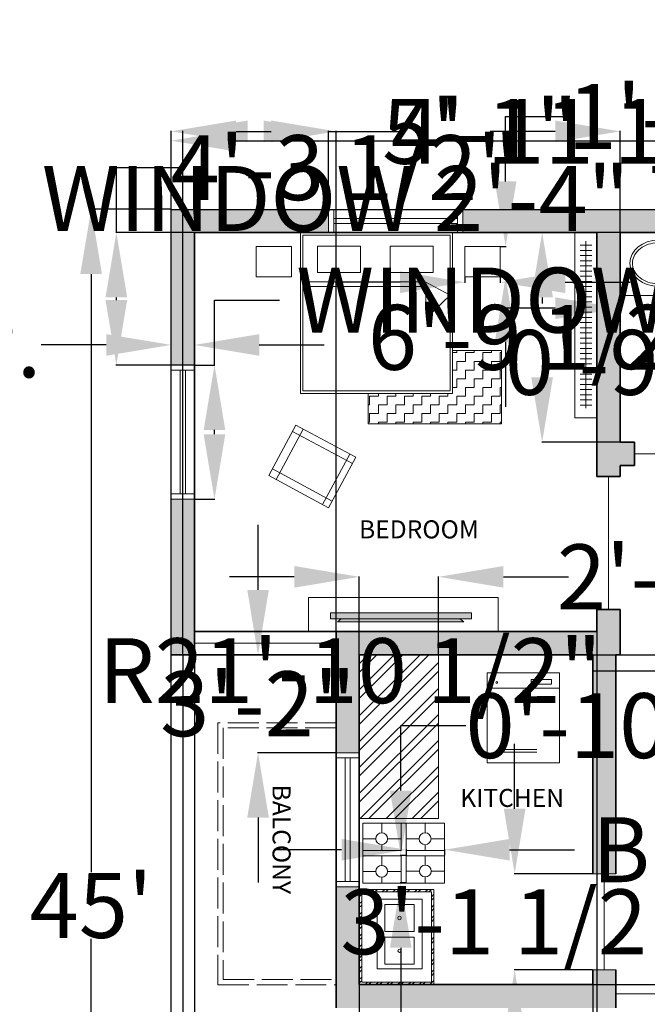
# Model space of a CAD drawing. Units: inches. Extents: x 29 to 6336, y 3 to 2592.
# Tile 3 of 8: x 5288 to 5531, y 2184 to 2566. Entities that reach past the tile are written whole.
import ezdxf

# ---------------------------------------------------------------- set-up
doc = ezdxf.new("R2010")
doc.units = ezdxf.units.IN
doc.header["$MEASUREMENT"] = 0
doc.linetypes.add('ACAD_ISO02W100', pattern=[15, 12, -3])
for name, color, linetype, lineweight in [('A-ANNO-DIMS', 2, 'Continuous', 18), ('A-AREA-IDEN', 7, 'Continuous', 18), ('A-DOOR', 4, 'Continuous', 18), ('A-EQPM', 9, 'Continuous', 18), ('A-FLOR-CASE', 8, 'Continuous', 18), ('A-FLOR-FIXT', 8, 'Continuous', 18), ('A-FLOR-FIXT-PATT', 9, 'Continuous', 13), ('A-FLOR-OVHD', 8, 'ACAD_ISO02W100', 18), ('A-FLOR-PATT', 9, 'Continuous', 13), ('A-FURN', 8, 'Continuous', 18), ('A-FURN-PATT', 18, 'Continuous', 13), ('A-GLAZ', 116, 'Continuous', 18), ('A-WALL', 7, 'Continuous', 35), ('A-WALL-HIDN', 7, 'ACAD_ISO02W100', 18), ('A-WALL-PATT', 242, 'Continuous', 13), ('C-PROP', 7, 'Continuous', 25)]:
    doc.layers.add(name, color=color, linetype=linetype, lineweight=lineweight)
doc.styles.get("Standard").update_dxf_attribs({"font": 'arial.ttf'})
doc.dimstyles.get("Standard").update_dxf_attribs({"dimtxt": 25.18, "dimasz": 25.18, "dimexe": 0.18, "dimexo": 0.0625, "dimgap": 0.09, "dimtad": 0, "dimtih": 1, "dimtoh": 1, "dimdec": 0, "dimzin": 0, "dimdsep": 46, "dimlunit": 3, "dimtxsty": 'Standard', "dimcen": 0.09, "dimadec": 0, "dimazin": 0, "dimtfac": 1, "dimtdec": 0, "dimtofl": 0, "dimtmove": 0, "dimatfit": 3, "dimfxl": 1, "dimtolj": 1, "dimtzin": 0, "dimarcsym": 0})

# ---------------------------------------------------------------- blocks, each defined once
blk = doc.blocks.new('*D5')
at = {"layer": 'A-ANNO-DIMS', "color": 0, "lineweight": -2, "transparency": 16777216}
for p, q in [((5346.66, 2492.39), (5346.66, 2519.15)), ((5371.84, 2518.97), (5594.69, 2518.97)), ((5861.48, 2518.97), (5638.62, 2518.97)), ((5886.66, 2492.39), (5886.66, 2519.15))]:
    blk.add_line(p, q, dxfattribs=at)
at = {"layer": 'A-ANNO-DIMS', "color": 0, "transparency": 16777216}
for points in [[(5371.84, 2523.17), (5371.84, 2514.77), (5346.66, 2518.97)], [(5861.48, 2523.17), (5861.48, 2514.77), (5886.66, 2518.97)]]:
    blk.add_solid(points, dxfattribs=at)
at = {"layer": 'Defpoints', "color": 0, "transparency": 16777216}
for p in [(5886.66, 2518.97), (5346.66, 2492.33), (5886.66, 2492.33)]:
    blk.add_point(p, dxfattribs=at)
at = {"layer": 'A-ANNO-DIMS', "color": 0, "transparency": 16777216, "insert": (5616.66, 2518.97), "char_height": 25.18, "attachment_point": 5}
blk.add_mtext("\\A1;45'", dxfattribs=at)
blk = doc.blocks.new('*D6')
at = {"layer": 'A-ANNO-DIMS', "color": 0, "lineweight": -2, "transparency": 16777216}
for p, q in [((5346.6, 2492.39), (5315.46, 2492.39)), ((5315.64, 2467.21), (5315.64, 2235.26)), ((5315.64, 1977.51), (5315.64, 2209.47)), ((5346.6, 1952.33), (5315.46, 1952.33))]:
    blk.add_line(p, q, dxfattribs=at)
at = {"layer": 'A-ANNO-DIMS', "color": 0, "transparency": 16777216}
for points in [[(5311.44, 2467.21), (5319.83, 2467.21), (5315.64, 2492.39)], [(5311.44, 1977.51), (5319.83, 1977.51), (5315.64, 1952.33)]]:
    blk.add_solid(points, dxfattribs=at)
at = {"layer": 'Defpoints', "color": 0, "transparency": 16777216}
for p in [(5346.66, 2492.39), (5315.64, 1952.33), (5346.66, 1952.33)]:
    blk.add_point(p, dxfattribs=at)
at = {"layer": 'A-ANNO-DIMS', "color": 0, "transparency": 16777216, "insert": (5315.64, 2222.36), "char_height": 25.18, "attachment_point": 5}
blk.add_mtext("\\A1;45'", dxfattribs=at)
blk = doc.blocks.new('WIN-48')
for p, q in [((0, 9), (0, 0)), ((2, 9), (2, 0)), ((50, 9), (50, 0)), ((52, 9), (52, 0)), ((2, 5.5), (50, 5.5)), ((2, 3.5), (50, 3.5))]:
    blk.add_line(p, q)
blk = doc.blocks.new('BASIN-VANITY')
for p, q in [((32.36, 0), (32.36, 24.47)), ((0, 0), (32.36, 0))]:
    blk.add_line(p, q)
blk.add_circle((14.85, 12.56), 0.667)
blk.add_ellipse((14.85, 12.56), major_axis=(11.1, 0), ratio=0.808824)
blk.add_open_spline([(24.95, 12.56), (24.95, 13.21), (24.85, 13.86), (24.35, 15.41), (23.86, 16.28), (22.49, 17.85), (21.62, 18.55), (19.61, 19.66), (18.47, 20.07), (16.07, 20.54), (14.82, 20.6), (12.37, 20.35), (11.18, 20.05), (9.01, 19.14), (8.04, 18.52), (6.44, 17.08), (5.81, 16.25), (4.97, 14.49), (4.75, 13.56), (4.73, 11.7), (4.93, 10.77), (5.73, 9), (6.33, 8.16), (7.89, 6.69), (8.85, 6.07), (10.99, 5.12), (12.18, 4.8), (14.62, 4.52), (15.88, 4.56), (18.29, 4.99), (19.44, 5.38), (21.47, 6.46), (22.36, 7.14), (23.77, 8.7), (24.29, 9.57), (24.83, 11.15), (24.95, 11.85), (24.95, 12.56)], degree=3, knots=[0, 0, 0, 0, 0.253102, 0.253102, 0.612978, 0.612978, 0.972853, 0.972853, 1.332728, 1.332728, 1.692603, 1.692603, 2.052478, 2.052478, 2.412354, 2.412354, 2.772229, 2.772229, 3.132104, 3.132104, 3.491979, 3.491979, 3.851854, 3.851854, 4.21173, 4.21173, 4.571605, 4.571605, 4.93148, 4.93148, 5.291355, 5.291355, 5.651231, 5.651231, 6.011106, 6.011106, 6.283185, 6.283185, 6.283185, 6.283185])
blk = doc.blocks.new('COOKTOP-BURNER')
for p, q in [((7.29, 6.87), (7.29, 10.62)), ((5, 4.58), (0, 4.58)), ((9.59, 4.58), (14.83, 4.58)), ((7.29, 2.28), (7.29, 0))]:
    blk.add_line(p, q)
blk.add_circle((7.29, 4.58), 2.3)
blk = doc.blocks.new('NIGHTSTAND-14X12')
blk.add_lwpolyline([(0, 11.85), (13.72, 11.85), (13.72, 0), (0, 0)], close=True)
blk = doc.blocks.new('*D22')
at = {"layer": 'A-ANNO-DIMS', "color": 0, "lineweight": -2, "transparency": 16777216}
for p, q in [((5363.46, 2431.95), (5363.46, 2457.13)), ((5363.46, 2457.13), (5388.64, 2457.13)), ((5355.72, 2431.95), (5363.64, 2431.95)), ((5363.46, 2405.13), (5363.46, 2406.77)), ((5355.72, 2379.95), (5363.64, 2379.95))]:
    blk.add_line(p, q, dxfattribs=at)
at = {"layer": 'A-ANNO-DIMS', "color": 0, "transparency": 16777216}
for points in [[(5359.26, 2406.77), (5367.65, 2406.77), (5363.46, 2431.95)], [(5359.26, 2405.13), (5367.65, 2405.13), (5363.46, 2379.95)]]:
    blk.add_solid(points, dxfattribs=at)
at = {"layer": 'Defpoints', "color": 0, "transparency": 16777216}
for p in [(5355.66, 2431.95), (5363.46, 2431.95), (5355.66, 2379.95)]:
    blk.add_point(p, dxfattribs=at)
at = {"layer": 'A-ANNO-DIMS', "color": 0, "transparency": 16777216, "insert": (5548.04, 2457.13), "char_height": 25.18, "attachment_point": 5}
blk.add_mtext('\\A1;WINDOW 4\'-4" TYP.', dxfattribs=at)
blk = doc.blocks.new('*D23')
at = {"layer": 'A-ANNO-DIMS', "color": 0, "lineweight": -2, "transparency": 16777216}
for p, q in [((5321.48, 2439.75), (5296.3, 2439.75)), ((5346.66, 2432.01), (5346.66, 2439.93)), ((5355.66, 2432.01), (5355.66, 2439.93)), ((5380.84, 2439.75), (5406.02, 2439.75))]:
    blk.add_line(p, q, dxfattribs=at)
at = {"layer": 'A-ANNO-DIMS', "color": 0, "transparency": 16777216}
for points in [[(5321.48, 2443.94), (5321.48, 2435.55), (5346.66, 2439.75)], [(5380.84, 2443.94), (5380.84, 2435.55), (5355.66, 2439.75)]]:
    blk.add_solid(points, dxfattribs=at)
at = {"layer": 'Defpoints', "color": 0, "transparency": 16777216}
for p in [(5346.66, 2439.75), (5346.66, 2431.95), (5355.66, 2431.95)]:
    blk.add_point(p, dxfattribs=at)
at = {"layer": 'A-ANNO-DIMS', "color": 0, "transparency": 16777216, "insert": (5219.47, 2439.75), "char_height": 25.18, "attachment_point": 5}
blk.add_mtext('\\A1;0\'-9" TYP.', dxfattribs=at)
blk = doc.blocks.new('*D24')
at = {"layer": 'A-ANNO-DIMS', "color": 0, "lineweight": -2, "transparency": 16777216}
for p, q in [((5412.73, 2243.97), (5387.55, 2243.97)), ((5437.91, 2241.81), (5437.91, 2244.15)), ((5452.73, 2241.81), (5452.73, 2244.15)), ((5477.91, 2243.97), (5503.09, 2243.97))]:
    blk.add_line(p, q, dxfattribs=at)
at = {"layer": 'A-ANNO-DIMS', "color": 0, "transparency": 16777216}
for points in [[(5412.73, 2248.16), (5412.73, 2239.77), (5437.91, 2243.97)], [(5477.91, 2248.16), (5477.91, 2239.77), (5452.73, 2243.97)]]:
    blk.add_solid(points, dxfattribs=at)
at = {"layer": 'Defpoints', "color": 0, "transparency": 16777216}
for p in [(5437.91, 2241.74), (5452.73, 2243.97), (5452.73, 2241.74)]:
    blk.add_point(p, dxfattribs=at)
at = {"layer": 'A-ANNO-DIMS', "color": 0, "transparency": 16777216, "insert": (5658.52, 2243.97), "char_height": 25.18, "attachment_point": 5}
blk.add_mtext('\\A1;BURNER 1\'-3" TYP.', dxfattribs=at)
blk = doc.blocks.new('*D25')
at = {"layer": 'A-ANNO-DIMS', "color": 0, "lineweight": -2, "transparency": 16777216}
for p, q in [((5435.68, 2266.92), (5435.68, 2292.1)), ((5435.68, 2292.1), (5460.86, 2292.1)), ((5437.84, 2241.74), (5435.5, 2241.74)), ((5437.84, 2231.12), (5435.5, 2231.12)), ((5435.68, 2205.94), (5435.68, 2180.76))]:
    blk.add_line(p, q, dxfattribs=at)
at = {"layer": 'A-ANNO-DIMS', "color": 0, "transparency": 16777216}
for points in [[(5431.49, 2266.92), (5439.88, 2266.92), (5435.68, 2241.74)], [(5431.49, 2205.94), (5439.88, 2205.94), (5435.68, 2231.12)]]:
    blk.add_solid(points, dxfattribs=at)
at = {"layer": 'Defpoints', "color": 0, "transparency": 16777216}
for p in [(5435.68, 2241.74), (5437.91, 2241.74), (5437.91, 2231.12)]:
    blk.add_point(p, dxfattribs=at)
at = {"layer": 'A-ANNO-DIMS', "color": 0, "transparency": 16777216, "insert": (5576.81, 2292.1), "char_height": 25.18, "attachment_point": 5}
blk.add_mtext('\\A1;0\'-10 1/2" TYP.', dxfattribs=at)
blk = doc.blocks.new('*D26')
at = {"layer": 'A-ANNO-DIMS', "color": 0, "lineweight": -2, "transparency": 16777216}
for p, q in [((5633.95, 2496.53), (5608.77, 2496.53)), ((5659.13, 2492.39), (5659.13, 2496.71)), ((5687.13, 2492.39), (5687.13, 2496.71)), ((5712.31, 2496.53), (5737.49, 2496.53))]:
    blk.add_line(p, q, dxfattribs=at)
at = {"layer": 'A-ANNO-DIMS', "color": 0, "transparency": 16777216}
for points in [[(5633.95, 2500.73), (5633.95, 2492.33), (5659.13, 2496.53)], [(5712.31, 2500.73), (5712.31, 2492.33), (5687.13, 2496.53)]]:
    blk.add_solid(points, dxfattribs=at)
at = {"layer": 'Defpoints', "color": 0, "transparency": 16777216}
for p in [(5659.13, 2496.53), (5659.13, 2492.33), (5687.13, 2492.33)]:
    blk.add_point(p, dxfattribs=at)
at = {"layer": 'A-ANNO-DIMS', "color": 0, "transparency": 16777216, "insert": (5449.36, 2496.53), "char_height": 25.18, "attachment_point": 5}
blk.add_mtext('\\A1;WINDOW 2\'-4" TYP.', dxfattribs=at)
blk = doc.blocks.new('*D27')
at = {"layer": 'A-ANNO-DIMS', "color": 0, "lineweight": -2, "transparency": 16777216}
for p, q in [((5654.93, 2517.51), (5654.93, 2542.69)), ((5659.07, 2492.33), (5654.75, 2492.33)), ((5659.07, 2483.33), (5654.75, 2483.33)), ((5654.93, 2458.15), (5654.93, 2432.97)), ((5654.93, 2432.97), (5629.75, 2432.97))]:
    blk.add_line(p, q, dxfattribs=at)
at = {"layer": 'A-ANNO-DIMS', "color": 0, "transparency": 16777216}
for points in [[(5650.73, 2517.51), (5659.12, 2517.51), (5654.93, 2492.33)], [(5650.73, 2458.15), (5659.12, 2458.15), (5654.93, 2483.33)]]:
    blk.add_solid(points, dxfattribs=at)
at = {"layer": 'Defpoints', "color": 0, "transparency": 16777216}
for p in [(5659.13, 2492.33), (5654.93, 2483.33), (5659.13, 2483.33)]:
    blk.add_point(p, dxfattribs=at)
at = {"layer": 'A-ANNO-DIMS', "color": 0, "transparency": 16777216, "insert": (5552.92, 2432.97), "char_height": 25.18, "attachment_point": 5}
blk.add_mtext('\\A1;0\'-9" TYP.', dxfattribs=at)
blk = doc.blocks.new('*D36')
at = {"layer": 'A-ANNO-DIMS', "color": 0, "lineweight": -2, "transparency": 16777216}
for p, q in [((5520.77, 2458.79), (5520.77, 2453.82)), ((5553.13, 2458.79), (5553.13, 2453.82)), ((5495.59, 2454), (5470.41, 2454)), ((5578.31, 2454), (5603.49, 2454))]:
    blk.add_line(p, q, dxfattribs=at)
at = {"layer": 'A-ANNO-DIMS', "color": 0, "transparency": 16777216}
for points in [[(5495.59, 2458.2), (5495.59, 2449.81), (5520.77, 2454)], [(5578.31, 2458.2), (5578.31, 2449.81), (5553.13, 2454)]]:
    blk.add_solid(points, dxfattribs=at)
at = {"layer": 'Defpoints', "color": 0, "transparency": 16777216}
for p in [(5520.77, 2458.86), (5553.13, 2458.86), (5553.13, 2454)]:
    blk.add_point(p, dxfattribs=at)
at = {"layer": 'A-ANNO-DIMS', "color": 0, "transparency": 16777216, "insert": (5778.73, 2454), "char_height": 25.18, "attachment_point": 5}
blk.add_mtext('\\A1;VANITY 2\'-8 1/2" TYP.', dxfattribs=at)
blk = doc.blocks.new('*D40')
at = {"layer": 'A-ANNO-DIMS', "color": 0, "lineweight": -2, "transparency": 16777216}
for p, q in [((5435.4, 2464.07), (5410.22, 2464.07)), ((5460.58, 2466.07), (5460.58, 2463.89)), ((5474.29, 2466.07), (5474.29, 2463.89)), ((5499.47, 2464.07), (5524.65, 2464.07))]:
    blk.add_line(p, q, dxfattribs=at)
at = {"layer": 'A-ANNO-DIMS', "color": 0, "transparency": 16777216}
for points in [[(5435.4, 2468.27), (5435.4, 2459.88), (5460.58, 2464.07)], [(5499.47, 2468.27), (5499.47, 2459.88), (5474.29, 2464.07)]]:
    blk.add_solid(points, dxfattribs=at)
at = {"layer": 'Defpoints', "color": 0, "transparency": 16777216}
for p in [(5460.58, 2466.13), (5474.29, 2466.13), (5474.29, 2464.07)]:
    blk.add_point(p, dxfattribs=at)
at = {"layer": 'A-ANNO-DIMS', "color": 0, "transparency": 16777216, "insert": (5749.42, 2464.07), "char_height": 25.18, "attachment_point": 5}
blk.add_mtext('\\A1;NIGHTSTAND 1\'-1 1/2" TYP.', dxfattribs=at)
blk = doc.blocks.new('*D41')
at = {"layer": 'A-ANNO-DIMS', "color": 0, "lineweight": -2, "transparency": 16777216}
for p, q in [((5476.35, 2503.16), (5476.35, 2528.34)), ((5476.35, 2528.34), (5501.53, 2528.34)), ((5474.36, 2477.98), (5476.53, 2477.98)), ((5474.36, 2466.13), (5476.53, 2466.13)), ((5476.35, 2440.95), (5476.35, 2415.77))]:
    blk.add_line(p, q, dxfattribs=at)
at = {"layer": 'A-ANNO-DIMS', "color": 0, "transparency": 16777216}
for points in [[(5472.16, 2503.16), (5480.55, 2503.16), (5476.35, 2477.98)], [(5472.16, 2440.95), (5480.55, 2440.95), (5476.35, 2466.13)]]:
    blk.add_solid(points, dxfattribs=at)
at = {"layer": 'Defpoints', "color": 0, "transparency": 16777216}
for p in [(5474.29, 2477.98), (5476.35, 2477.98), (5474.29, 2466.13)]:
    blk.add_point(p, dxfattribs=at)
at = {"layer": 'A-ANNO-DIMS', "color": 0, "transparency": 16777216, "insert": (5577.18, 2528.34), "char_height": 25.18, "attachment_point": 5}
blk.add_mtext('\\A1;1\'-0" TYP.', dxfattribs=at)
blk = doc.blocks.new('*D42')
at = {"layer": 'A-ANNO-DIMS', "color": 0, "lineweight": -2, "transparency": 16777216}
for p, q in [((5511.77, 2337.07), (5511.77, 1921.9)), ((5355.66, 2328.5), (5355.66, 1921.9)), ((5380.84, 1922.08), (5391.56, 1922.08)), ((5486.59, 1922.08), (5475.87, 1922.08))]:
    blk.add_line(p, q, dxfattribs=at)
at = {"layer": 'A-ANNO-DIMS', "color": 0, "transparency": 16777216}
for points in [[(5380.84, 1926.28), (5380.84, 1917.88), (5355.66, 1922.08)], [(5486.59, 1926.28), (5486.59, 1917.88), (5511.77, 1922.08)]]:
    blk.add_solid(points, dxfattribs=at)
at = {"layer": 'Defpoints', "color": 0, "transparency": 16777216}
for p in [(5511.77, 2337.13), (5355.66, 2328.56), (5511.77, 1922.08)]:
    blk.add_point(p, dxfattribs=at)
at = {"layer": 'A-ANNO-DIMS', "color": 0, "transparency": 16777216, "insert": (5433.71, 1922.08), "char_height": 25.18, "attachment_point": 5}
blk.add_mtext('\\A1;13\'-0"', dxfattribs=at)
blk = doc.blocks.new('*D43')
at = {"layer": 'A-ANNO-DIMS', "color": 0, "lineweight": -2, "transparency": 16777216}
for p, q in [((5495.59, 2522.58), (5470.41, 2522.58)), ((5520.77, 2483.39), (5520.77, 2522.76)), ((5624.6, 2483.39), (5624.6, 2522.76)), ((5649.78, 2522.58), (5674.96, 2522.58))]:
    blk.add_line(p, q, dxfattribs=at)
at = {"layer": 'A-ANNO-DIMS', "color": 0, "transparency": 16777216}
for points in [[(5495.59, 2526.78), (5495.59, 2518.38), (5520.77, 2522.58)], [(5649.78, 2526.78), (5649.78, 2518.38), (5624.6, 2522.58)]]:
    blk.add_solid(points, dxfattribs=at)
at = {"layer": 'Defpoints', "color": 0, "transparency": 16777216}
for p in [(5624.6, 2522.58), (5520.77, 2483.33), (5624.6, 2483.33)]:
    blk.add_point(p, dxfattribs=at)
at = {"layer": 'A-ANNO-DIMS', "color": 0, "transparency": 16777216, "insert": (5572.68, 2522.58), "char_height": 25.18, "attachment_point": 5}
blk.add_mtext('\\A1;8\'-8"', dxfattribs=at)
blk = doc.blocks.new('*D47')
at = {"layer": 'A-ANNO-DIMS', "color": 0, "lineweight": -2, "transparency": 16777216}
for p, q in [((5520.71, 2483.33), (5490.34, 2483.33)), ((5490.52, 2458.15), (5490.52, 2455.8)), ((5490.52, 2427.23), (5490.52, 2429.58)), ((5520.71, 2402.05), (5490.34, 2402.05))]:
    blk.add_line(p, q, dxfattribs=at)
at = {"layer": 'A-ANNO-DIMS', "color": 0, "transparency": 16777216}
for points in [[(5486.32, 2458.15), (5494.72, 2458.15), (5490.52, 2483.33)], [(5486.32, 2427.23), (5494.72, 2427.23), (5490.52, 2402.05)]]:
    blk.add_solid(points, dxfattribs=at)
at = {"layer": 'Defpoints', "color": 0, "transparency": 16777216}
for p in [(5490.52, 2483.33), (5520.77, 2483.33), (5520.77, 2402.05)]:
    blk.add_point(p, dxfattribs=at)
at = {"layer": 'A-ANNO-DIMS', "color": 0, "transparency": 16777216, "insert": (5490.52, 2442.69), "char_height": 25.18, "attachment_point": 5}
blk.add_mtext('\\A1;6\'-9 1/2"', dxfattribs=at)
blk = doc.blocks.new('*D48')
at = {"layer": 'A-ANNO-DIMS', "color": 0, "lineweight": -2, "transparency": 16777216}
for p, q in [((5351.16, 2319.63), (5351.16, 2522.76)), ((5376.34, 2522.58), (5385.42, 2522.58)), ((5410.6, 2319.63), (5410.6, 2522.76)), ((5410.6, 2522.58), (5435.78, 2522.58))]:
    blk.add_line(p, q, dxfattribs=at)
at = {"layer": 'A-ANNO-DIMS', "color": 0, "transparency": 16777216}
for points in [[(5376.34, 2526.78), (5376.34, 2518.38), (5351.16, 2522.58)], [(5385.42, 2526.78), (5385.42, 2518.38), (5410.6, 2522.58)]]:
    blk.add_solid(points, dxfattribs=at)
at = {"layer": 'Defpoints', "color": 0, "transparency": 16777216}
for p in [(5410.6, 2522.58), (5351.16, 2319.56), (5410.6, 2319.56)]:
    blk.add_point(p, dxfattribs=at)
at = {"layer": 'A-ANNO-DIMS', "color": 0, "transparency": 16777216, "insert": (5508.96, 2522.58), "char_height": 25.18, "attachment_point": 5}
blk.add_mtext('\\A1;4\'-11 1/2"', dxfattribs=at)
blk = doc.blocks.new('*D49')
at = {"layer": 'A-ANNO-DIMS', "color": 0, "lineweight": -2, "transparency": 16777216}
for p, q in [((5419.6, 2191.59), (5419.6, 1921.9)), ((5510.11, 2191.59), (5510.11, 1921.9)), ((5444.78, 1922.08), (5484.93, 1922.08)), ((5510.11, 1922.08), (5535.29, 1922.08))]:
    blk.add_line(p, q, dxfattribs=at)
at = {"layer": 'A-ANNO-DIMS', "color": 0, "transparency": 16777216}
for points in [[(5444.78, 1926.28), (5444.78, 1917.88), (5419.6, 1922.08)], [(5484.93, 1926.28), (5484.93, 1917.88), (5510.11, 1922.08)]]:
    blk.add_solid(points, dxfattribs=at)
at = {"layer": 'Defpoints', "color": 0, "transparency": 16777216}
for p in [(5419.6, 2191.65), (5510.11, 2191.65), (5510.11, 1922.08)]:
    blk.add_point(p, dxfattribs=at)
at = {"layer": 'A-ANNO-DIMS', "color": 0, "transparency": 16777216, "insert": (5598.08, 1922.08), "char_height": 25.18, "attachment_point": 5}
blk.add_mtext('\\A1;7\'-6 1/2"', dxfattribs=at)
blk = doc.blocks.new('*D50')
at = {"layer": 'A-ANNO-DIMS', "color": 0, "lineweight": -2, "transparency": 16777216}
for p, q in [((5510.17, 2319.56), (5917.09, 2319.56)), ((5916.91, 2294.38), (5916.91, 2268.55)), ((5916.91, 2216.83), (5916.91, 2242.66)), ((5510.17, 2191.65), (5917.09, 2191.65))]:
    blk.add_line(p, q, dxfattribs=at)
at = {"layer": 'A-ANNO-DIMS', "color": 0, "transparency": 16777216}
for points in [[(5912.71, 2294.38), (5921.1, 2294.38), (5916.91, 2319.56)], [(5912.71, 2216.83), (5921.1, 2216.83), (5916.91, 2191.65)]]:
    blk.add_solid(points, dxfattribs=at)
at = {"layer": 'Defpoints', "color": 0, "transparency": 16777216}
for p in [(5510.11, 2319.56), (5916.91, 2319.56), (5510.11, 2191.65)]:
    blk.add_point(p, dxfattribs=at)
at = {"layer": 'A-ANNO-DIMS', "color": 0, "transparency": 16777216, "insert": (5916.91, 2255.61), "char_height": 25.18, "attachment_point": 5}
blk.add_mtext('\\A1;10\'-8"', dxfattribs=at)
blk = doc.blocks.new('*D62')
at = {"layer": 'A-ANNO-DIMS', "color": 0, "lineweight": -2, "transparency": 16777216}
for p, q in [((5346.66, 2492.39), (5346.66, 2522.76)), ((5371.84, 2522.58), (5382.53, 2522.58)), ((5407.71, 2492.39), (5407.71, 2522.76)), ((5407.71, 2522.58), (5432.89, 2522.58))]:
    blk.add_line(p, q, dxfattribs=at)
at = {"layer": 'A-ANNO-DIMS', "color": 0, "transparency": 16777216}
for points in [[(5371.84, 2526.78), (5371.84, 2518.38), (5346.66, 2522.58)], [(5382.53, 2526.78), (5382.53, 2518.38), (5407.71, 2522.58)]]:
    blk.add_solid(points, dxfattribs=at)
at = {"layer": 'Defpoints', "color": 0, "transparency": 16777216}
for p in [(5407.71, 2522.58), (5346.66, 2492.33), (5407.71, 2492.33)]:
    blk.add_point(p, dxfattribs=at)
at = {"layer": 'A-ANNO-DIMS', "color": 0, "transparency": 16777216, "insert": (5466.45, 2522.58), "char_height": 25.18, "attachment_point": 5}
blk.add_mtext('\\A1;5\'-1"', dxfattribs=at)
blk = doc.blocks.new('*D63')
at = {"layer": 'A-ANNO-DIMS', "color": 0, "lineweight": -2, "transparency": 16777216}
for p, q in [((5325.41, 2483.33), (5325.41, 2508.51)), ((5325.41, 2508.51), (5350.59, 2508.51)), ((5355.6, 2483.33), (5325.23, 2483.33)), ((5325.41, 2457.13), (5325.41, 2458.15)), ((5355.6, 2431.95), (5325.23, 2431.95))]:
    blk.add_line(p, q, dxfattribs=at)
at = {"layer": 'A-ANNO-DIMS', "color": 0, "transparency": 16777216}
for points in [[(5321.21, 2458.15), (5329.6, 2458.15), (5325.41, 2483.33)], [(5321.21, 2457.13), (5329.6, 2457.13), (5325.41, 2431.95)]]:
    blk.add_solid(points, dxfattribs=at)
at = {"layer": 'Defpoints', "color": 0, "transparency": 16777216}
for p in [(5325.41, 2483.33), (5355.66, 2483.33), (5355.66, 2431.95)]:
    blk.add_point(p, dxfattribs=at)
at = {"layer": 'A-ANNO-DIMS', "color": 0, "transparency": 16777216, "insert": (5413.99, 2508.51), "char_height": 25.18, "attachment_point": 5}
blk.add_mtext('\\A1;4\'-3 1/2"', dxfattribs=at)
blk = doc.blocks.new('*D68')
at = {"layer": 'A-ANNO-DIMS', "color": 0, "lineweight": -2, "transparency": 16777216}
for p, q in [((5479.86, 2259.85), (5479.86, 2285.03)), ((5510.05, 2234.67), (5479.68, 2234.67)), ((5510.05, 2197.33), (5479.68, 2197.33)), ((5479.86, 2172.15), (5479.86, 2146.97))]:
    blk.add_line(p, q, dxfattribs=at)
at = {"layer": 'A-ANNO-DIMS', "color": 0, "transparency": 16777216}
for points in [[(5475.66, 2259.85), (5484.06, 2259.85), (5479.86, 2234.67)], [(5475.66, 2172.15), (5484.06, 2172.15), (5479.86, 2197.33)]]:
    blk.add_solid(points, dxfattribs=at)
at = {"layer": 'Defpoints', "color": 0, "transparency": 16777216}
for p in [(5479.86, 2234.67), (5510.11, 2234.67), (5510.11, 2197.33)]:
    blk.add_point(p, dxfattribs=at)
at = {"layer": 'A-ANNO-DIMS', "color": 0, "transparency": 16777216, "insert": (5479.86, 2216), "char_height": 25.18, "attachment_point": 5}
blk.add_mtext('\\A1;3\'-1 1/2"', dxfattribs=at)
blk = doc.blocks.new('*D69')
at = {"layer": 'A-ANNO-DIMS', "color": 0, "lineweight": -2, "transparency": 16777216}
for p, q in [((5394.42, 2349.81), (5369.24, 2349.81)), ((5419.6, 2319.63), (5419.6, 2349.99)), ((5450.34, 2319.63), (5450.34, 2349.99)), ((5475.52, 2349.81), (5500.7, 2349.81))]:
    blk.add_line(p, q, dxfattribs=at)
at = {"layer": 'A-ANNO-DIMS', "color": 0, "transparency": 16777216}
for points in [[(5394.42, 2354.01), (5394.42, 2345.62), (5419.6, 2349.81)], [(5475.52, 2354.01), (5475.52, 2345.62), (5450.34, 2349.81)]]:
    blk.add_solid(points, dxfattribs=at)
at = {"layer": 'Defpoints', "color": 0, "transparency": 16777216}
for p in [(5450.34, 2349.81), (5419.6, 2319.56), (5450.34, 2319.56)]:
    blk.add_point(p, dxfattribs=at)
at = {"layer": 'A-ANNO-DIMS', "color": 0, "transparency": 16777216, "insert": (5563.81, 2349.81), "char_height": 25.18, "attachment_point": 5}
blk.add_mtext('\\A1;2\'-6 1/2"', dxfattribs=at)
blk = doc.blocks.new('*D70')
at = {"layer": 'A-ANNO-DIMS', "color": 0, "lineweight": -2, "transparency": 16777216}
for p, q in [((5380.35, 2344.74), (5380.35, 2369.92)), ((5410.54, 2319.56), (5380.17, 2319.56)), ((5410.54, 2281.61), (5380.17, 2281.61)), ((5380.35, 2256.43), (5380.35, 2231.25))]:
    blk.add_line(p, q, dxfattribs=at)
at = {"layer": 'A-ANNO-DIMS', "color": 0, "transparency": 16777216}
for points in [[(5376.16, 2344.74), (5384.55, 2344.74), (5380.35, 2319.56)], [(5376.16, 2256.43), (5384.55, 2256.43), (5380.35, 2281.61)]]:
    blk.add_solid(points, dxfattribs=at)
at = {"layer": 'Defpoints', "color": 0, "transparency": 16777216}
for p in [(5380.35, 2319.56), (5410.6, 2319.56), (5410.6, 2281.61)]:
    blk.add_point(p, dxfattribs=at)
at = {"layer": 'A-ANNO-DIMS', "color": 0, "transparency": 16777216, "insert": (5380.35, 2300.58), "char_height": 25.18, "attachment_point": 5}
blk.add_mtext('\\A1;3\'-2"', dxfattribs=at)
blk = doc.blocks.new('*D71')
at = {"layer": 'A-ANNO-DIMS', "color": 0, "lineweight": -2, "transparency": 16777216}
for p, q in [((5510.6, 2313.41), (5548.31, 2313.41)), ((5835.74, 2313.41), (5835.92, 2313.41)), ((5835.83, 2313.32), (5835.83, 2313.5))]:
    blk.add_line(p, q, dxfattribs=at)
at = {"layer": 'A-ANNO-DIMS', "color": 0, "transparency": 16777216}
blk.add_solid([(5548.31, 2317.61), (5548.31, 2309.22), (5573.49, 2313.41)], dxfattribs=at)
at = {"layer": 'Defpoints', "color": 0, "transparency": 16777216}
for p in [(5573.49, 2313.41), (5835.83, 2313.41)]:
    blk.add_point(p, dxfattribs=at)
at = {"layer": 'A-ANNO-DIMS', "color": 0, "transparency": 16777216, "insert": (5416.09, 2313.41), "char_height": 25.18, "attachment_point": 5}
blk.add_mtext('\\A1;R21\'-10 1/2"', dxfattribs=at)

msp = doc.modelspace()

# ---------------------------------------------------------------- hatches: boundary and pattern name
at = {"layer": 'A-FLOR-FIXT-PATT'}
h = msp.add_hatch(dxfattribs=at)
h.set_pattern_fill('ANSI32', color=256, scale=19)
h.paths.add_polyline_path([(5450.34, 2319.56), (5419.6, 2319.56), (5419.6, 2256.05), (5450.34, 2256.05)])
h = msp.add_hatch(dxfattribs=at)
h.set_pattern_fill('ANSI32', color=256, scale=7.9)
h.paths.add_polyline_path([(5448.57, 2228.6), (5419.6, 2228.6), (5419.6, 2191.65), (5448.57, 2191.65)])
h.paths.add_polyline_path([(5447.57, 2227.6), (5447.57, 2192.65), (5420.6, 2192.65), (5420.6, 2227.6)], flags=16)
h.paths.add_polyline_path([(5426.58, 2224.82), (5444.03, 2224.82), (5444.03, 2197.8), (5426.58, 2197.8)], flags=0)
h.paths.add_polyline_path([(5429.46, 2222.71), (5440.95, 2222.71), (5440.95, 2212.28), (5429.46, 2212.28)], flags=0)
h.paths.add_polyline_path([(5435.89, 2217.5, -1), (5434.52, 2217.5, -1)], flags=0)
h.paths.add_polyline_path([(5429.46, 2210), (5440.95, 2210), (5440.95, 2199.58), (5429.46, 2199.58)], flags=0)
h.paths.add_polyline_path([(5435.83, 2204.79, -1), (5434.58, 2204.79, -1)], flags=0)
at = {"layer": 'A-FLOR-PATT'}
h = msp.add_hatch(dxfattribs=at)
h.set_pattern_fill('ZIGZAG', color=256, scale=27)
h.set_pattern_definition([(0, (0, 0), (3.375, 3.375), [3.375, -3.375]), (90, (3.375, 0), (-3.375, 3.375), [3.375, -3.375])])
h.paths.add_polyline_path([(5474.78, 2437.64), (5455.81, 2437.64), (5455.81, 2420.96), (5423.07, 2420.96), (5423.07, 2409.18), (5474.78, 2409.18)])
at = {"layer": 'A-FURN-PATT'}
h = msp.add_hatch(color=256, dxfattribs=at)
h.dxf.hatch_style = 1
h.paths.add_polyline_path([(5463.07, 2335.79), (5408.39, 2335.79), (5408.39, 2333.5), (5463.07, 2333.5)])
h.paths.add_polyline_path([(5458.63, 2333.5), (5412.53, 2333.5), (5411.1, 2332.36), (5460.11, 2332.36)])
at = {"layer": 'A-WALL-PATT'}
h = msp.add_hatch(color=256, dxfattribs=at)
h.dxf.hatch_style = 1
h.paths.add_polyline_path([(5558.68, 2492.33), (5459.71, 2492.33), (5459.71, 2483.33), (5511.77, 2483.33), (5511.77, 2388.68), (5520.77, 2388.68), (5520.77, 2393.05), (5526.31, 2393.05), (5526.31, 2402.05), (5520.77, 2402.05), (5520.77, 2483.33), (5558.68, 2483.33)])
h.paths.add_polyline_path([(5659.13, 2492.33), (5586.68, 2492.33), (5586.68, 2483.33), (5624.6, 2483.33), (5624.6, 2402.05), (5562.29, 2402.05), (5562.29, 2393.05), (5676.48, 2393.05), (5676.48, 2402.05), (5633.6, 2402.05), (5633.6, 2422.71), (5633.6, 2483.33), (5659.13, 2483.33)])
h.paths.add_polyline_path([(5886.66, 2492.33), (5687.13, 2492.33), (5687.13, 2483.33), (5712.66, 2483.33), (5712.66, 2468.69), (5721.66, 2468.69), (5721.66, 2483.33), (5877.66, 2483.33), (5877.66, 2106.48), (5858.21, 2106.48), (5858.21, 2097.48), (5877.66, 2097.48), (5877.66, 1961.33), (5877.66, 1952.33), (5886.66, 1952.33)])
h.paths.add_polyline_path([(5721.66, 2416.69), (5712.66, 2416.69), (5712.66, 2402.05), (5709.45, 2402.05), (5709.45, 2393.05), (5712.66, 2393.05), (5712.66, 2386.01), (5721.66, 2386.01)], flags=17)
h.paths.add_polyline_path([(5355.66, 2483.33), (5407.71, 2483.33), (5407.71, 2492.33), (5346.66, 2492.33), (5346.66, 2431.95), (5355.66, 2431.95)])
h.paths.add_polyline_path([(5355.66, 2379.95), (5346.66, 2379.95), (5346.66, 2319.56), (5355.66, 2319.56), (5355.66, 2328.56)])
h.paths.add_polyline_path([(5520.77, 2337.13), (5511.77, 2337.13), (5511.77, 2328.56), (5410.6, 2328.56), (5410.6, 2319.56), (5410.6, 2281.61), (5419.6, 2281.61), (5419.6, 2319.56), (5510.11, 2319.56), (5510.11, 2234.67), (5519.11, 2234.67), (5519.11, 2319.56), (5520.77, 2319.56)])
h.paths.add_polyline_path([(5519.11, 2197.33), (5510.11, 2197.33), (5510.11, 2191.65), (5419.6, 2191.65), (5419.6, 2228.6), (5419.6, 2229.61), (5410.6, 2229.61), (5410.6, 2182.65), (5519.11, 2182.65)])
h.paths.add_polyline_path([(5712.66, 2193.6), (5592.36, 2193.6), (5592.36, 2182.65), (5624.77, 2182.65), (5633.77, 2182.65), (5712.66, 2182.65)])
h.paths.add_polyline_path([(5633.77, 2182.65), (5624.77, 2182.65), (5624.77, 2051.72), (5633.77, 2051.72), (5691.77, 2051.72), (5691.77, 2060.72), (5633.77, 2060.72)])
h.paths.add_polyline_path([(5810.76, 2097.48), (5830.21, 2097.48), (5830.21, 2106.48), (5810.76, 2106.48), (5810.76, 2182.65), (5817.87, 2182.65), (5817.87, 2193.6), (5783.59, 2193.6), (5783.59, 2182.65), (5801.76, 2182.65), (5801.76, 2060.72), (5743.77, 2060.72), (5743.77, 2051.72), (5810.76, 2051.72)], flags=17)
h.paths.add_polyline_path([(5721.66, 2319.56), (5877.66, 2319.56), (5877.66, 2328.56), (5721.66, 2328.56), (5721.66, 2335.85), (5712.66, 2335.85), (5712.66, 2319.56), (5712.66, 2182.65), (5726.12, 2182.65), (5726.12, 2193.6), (5721.66, 2193.6)], flags=17)
h.paths.add_polyline_path([(5631.73, 2431.78), (5711.31, 2431.78), (5711.31, 2446.2), (5631.73, 2446.2)], flags=9)

# ---------------------------------------------------------------- linework, layer by layer
at = {"layer": 'A-DOOR'}
for p, q in [((5526.31, 2397.55), (5562.29, 2397.55)), ((5516.27, 2388.68), (5516.27, 2337.13)), ((5355.66, 2324.06), (5410.6, 2324.06)), ((5514.61, 2234.67), (5514.61, 2197.33)), ((5592.36, 2188.13), (5519.11, 2188.13))]:
    msp.add_line(p, q, dxfattribs=at)
at = {"layer": 'A-EQPM'}
for p, q in [((5469.25, 2306.59), (5497.24, 2306.59)), ((5474.54, 2282.87), (5488.46, 2282.87)), ((5474.54, 2281.87), (5488.46, 2281.87)), ((5435.82, 2254.27), (5435.82, 2243.64)), ((5437.82, 2254.27), (5437.82, 2243.64)), ((5421, 2243.64), (5435.82, 2243.64)), ((5421, 2241.64), (5435.82, 2241.64)), ((5435.82, 2241.64), (5435.82, 2231.02)), ((5437.82, 2243.64), (5452.65, 2243.64)), ((5437.82, 2241.64), (5437.82, 2231.02)), ((5437.82, 2241.64), (5452.65, 2241.64))]:
    msp.add_line(p, q, dxfattribs=at)
for points in [[(5469.25, 2312.56), (5497.24, 2312.56), (5497.24, 2277.63), (5469.25, 2277.63)], [(5486.25, 2309.99), (5494.19, 2309.99), (5494.19, 2308.22), (5486.25, 2308.22)], [(5421, 2254.27), (5452.65, 2254.27), (5452.65, 2231.02), (5421, 2231.02)]]:
    msp.add_lwpolyline(points, close=True, dxfattribs=at)
msp.add_circle((5472.91, 2308.86), 0.345, dxfattribs=at)
at = {"layer": 'A-FLOR-CASE'}
for p, q in [((5503.13, 2483.33), (5503.13, 2447.46)), ((5505.3, 2478.41), (5509.75, 2478.41)), ((5507.46, 2480.05), (5507.46, 2450.17)), ((5505.3, 2476.41), (5509.75, 2476.41)), ((5505.3, 2474.41), (5509.75, 2474.41)), ((5505.3, 2472.41), (5509.75, 2472.41)), ((5505.3, 2470.41), (5509.75, 2470.41)), ((5505.3, 2468.41), (5509.75, 2468.41)), ((5505.3, 2466.41), (5509.75, 2466.41)), ((5505.3, 2464.41), (5509.75, 2464.41)), ((5505.3, 2462.41), (5509.75, 2462.41)), ((5505.3, 2460.41), (5509.75, 2460.41)), ((5505.3, 2458.41), (5509.75, 2458.41)), ((5505.3, 2456.41), (5509.75, 2456.41)), ((5505.3, 2454.41), (5509.75, 2454.41)), ((5505.3, 2452.41), (5509.75, 2452.41)), ((5505.3, 2450.41), (5509.75, 2450.41)), ((5505.3, 2448.41), (5509.75, 2448.41)), ((5507.46, 2450.17), (5507.46, 2415.23)), ((5503.13, 2447.46), (5503.13, 2411.43)), ((5505.3, 2446.41), (5509.75, 2446.41)), ((5505.3, 2444.41), (5509.75, 2444.41)), ((5505.3, 2442.41), (5509.75, 2442.41)), ((5505.3, 2440.41), (5509.75, 2440.41)), ((5505.3, 2438.41), (5509.75, 2438.41)), ((5505.3, 2436.41), (5509.75, 2436.41)), ((5505.3, 2434.41), (5509.75, 2434.41)), ((5505.3, 2432.41), (5509.75, 2432.41)), ((5505.3, 2430.41), (5509.75, 2430.41)), ((5505.3, 2428.41), (5509.75, 2428.41)), ((5505.3, 2426.41), (5509.75, 2426.41)), ((5505.3, 2424.41), (5509.75, 2424.41)), ((5505.3, 2422.41), (5509.75, 2422.41)), ((5505.3, 2420.41), (5509.75, 2420.41)), ((5505.3, 2418.41), (5509.75, 2418.41)), ((5505.3, 2416.41), (5509.75, 2416.41)), ((5503.13, 2411.43), (5511.77, 2411.43))]:
    msp.add_line(p, q, dxfattribs=at)
at = {"layer": 'A-FLOR-FIXT'}
for points in [[(5419.6, 2319.56), (5450.34, 2319.56), (5450.34, 2256.05), (5419.6, 2256.05)], [(5419.6, 2228.6), (5448.57, 2228.6), (5448.57, 2191.65), (5419.6, 2191.65)], [(5420.6, 2227.6), (5447.57, 2227.6), (5447.57, 2192.65), (5420.6, 2192.65)], [(5426.58, 2224.82), (5444.03, 2224.82), (5444.03, 2197.8), (5426.58, 2197.8)], [(5429.46, 2222.71), (5440.95, 2222.71), (5440.95, 2212.28), (5429.46, 2212.28)], [(5429.46, 2210), (5440.95, 2210), (5440.95, 2199.58), (5429.46, 2199.58)]]:
    msp.add_lwpolyline(points, close=True, dxfattribs=at)
for centre, radius in [((5435.2, 2217.5), 0.682), ((5435.2, 2204.79), 0.623)]:
    msp.add_circle(centre, radius, dxfattribs=at)
at = {"layer": 'A-FLOR-OVHD'}
for p, q in [((5410.6, 2293.2), (5364.82, 2293.2)), ((5364.82, 2293.2), (5364.82, 2191.58)), ((5410.6, 2291.2), (5366.82, 2291.2)), ((5366.82, 2291.2), (5366.82, 2193.58)), ((5366.82, 2193.58), (5410.6, 2193.58)), ((5364.82, 2191.58), (5410.6, 2191.58))]:
    msp.add_line(p, q, dxfattribs=at)
at = {"layer": 'A-FLOR-PATT'}
for p, q in [((5455.81, 2437.64), (5455.81, 2437.64)), ((5455.81, 2437.64), (5474.78, 2437.64)), ((5474.78, 2437.64), (5474.78, 2409.18)), ((5423.07, 2409.18), (5423.07, 2420.96)), ((5474.78, 2409.18), (5423.07, 2409.18))]:
    msp.add_line(p, q, dxfattribs=at)
at = {"layer": 'A-FURN'}
for p, q in [((5397.77, 2464.26), (5445.2, 2464.26)), ((5445.2, 2464.26), (5454.81, 2459.01)), ((5445.65, 2450.31), (5445.2, 2464.26)), ((5397.77, 2462.4), (5445.26, 2462.36)), ((5454.81, 2459.01), (5445.65, 2450.31)), ((5387.35, 2387.52), (5397.9, 2407.14)), ((5393.73, 2406.23), (5416.94, 2393.74)), ((5415.91, 2397.45), (5405.36, 2377.83)), ((5385.9, 2391.66), (5409.11, 2379.17)), ((5412.53, 2333.5), (5411.1, 2332.36)), ((5460.11, 2332.36), (5458.63, 2333.5)), ((5411.1, 2332.36), (5460.11, 2332.36))]:
    msp.add_line(p, q, dxfattribs=at)
for points in [[(5396.77, 2483.33), (5455.81, 2483.33), (5455.81, 2420.96), (5396.77, 2420.96)], [(5397.77, 2482.33), (5454.81, 2482.33), (5454.81, 2421.96), (5397.77, 2421.96)], [(5403.46, 2478.09), (5420.07, 2478.09), (5420.07, 2467.84), (5403.46, 2467.84)], [(5431.6, 2478.09), (5448.2, 2478.09), (5448.2, 2467.84), (5431.6, 2467.84)], [(5395.05, 2408.67), (5418.26, 2396.19), (5407.71, 2376.57), (5384.49, 2389.05)], [(5399.87, 2328.56), (5473.5, 2328.56), (5473.5, 2341.86), (5399.87, 2341.86)], [(5408.39, 2333.5), (5463.07, 2333.5), (5463.07, 2335.79), (5408.39, 2335.79)]]:
    msp.add_lwpolyline(points, close=True, dxfattribs=at)
at = {"layer": 'A-GLAZ'}
for p, q in [((5407.71, 2483.33), (5407.71, 2492.33)), ((5409.71, 2483.33), (5409.71, 2492.33)), ((5457.71, 2483.33), (5457.71, 2492.33)), ((5459.71, 2483.33), (5459.71, 2492.33)), ((5409.71, 2488.83), (5457.71, 2488.83)), ((5409.71, 2488.83), (5457.71, 2488.83)), ((5409.71, 2486.83), (5457.71, 2486.83))]:
    msp.add_line(p, q, dxfattribs=at)
at = {"layer": 'A-WALL'}
for p, q in [((5355.66, 2483.33), (5511.77, 2483.33)), ((5355.66, 2328.56), (5355.66, 2483.33)), ((5511.77, 2388.68), (5511.77, 2483.33)), ((5520.77, 2402.05), (5520.77, 2483.33)), ((5520.77, 2483.33), (5624.6, 2483.33)), ((5520.77, 2402.05), (5526.31, 2402.05)), ((5526.31, 2402.05), (5526.31, 2393.05)), ((5520.77, 2393.05), (5526.31, 2393.05)), ((5520.77, 2388.68), (5520.77, 2393.05)), ((5520.77, 2388.68), (5511.77, 2388.68)), ((5511.77, 2328.56), (5511.77, 2337.13)), ((5511.77, 2337.13), (5520.77, 2337.13)), ((5520.77, 2319.56), (5520.77, 2337.13)), ((5355.66, 2328.56), (5511.77, 2328.56)), ((5355.66, 2328.56), (5355.66, 2319.56)), ((5410.6, 2319.56), (5410.6, 2328.56)), ((5355.66, 2319.56), (5346.66, 2319.56)), ((5355.66, 2319.56), (5410.6, 2319.56)), ((5410.6, 2182.65), (5410.6, 2319.56)), ((5419.6, 2191.65), (5419.6, 2319.56)), ((5419.6, 2319.56), (5510.11, 2319.56)), ((5510.11, 2234.67), (5510.11, 2319.56)), ((5519.11, 2319.56), (5520.77, 2319.56)), ((5519.11, 2234.67), (5519.11, 2319.56)), ((5510.11, 2191.65), (5510.11, 2197.33)), ((5519.11, 2182.65), (5519.11, 2197.33)), ((5419.6, 2191.65), (5510.11, 2191.65))]:
    msp.add_line(p, q, dxfattribs=at)
at = {"layer": 'A-WALL-HIDN'}
for p, q in [((5510.11, 2234.67), (5519.11, 2234.67)), ((5510.11, 2197.33), (5519.11, 2197.33))]:
    msp.add_line(p, q, dxfattribs=at)
at = {"layer": 'C-PROP'}
for p, q in [((5346.66, 1952.33), (5346.66, 2492.33)), ((5346.66, 2492.33), (5886.66, 2492.33)), ((5351.16, 2319.56), (5351.16, 1964.19))]:
    msp.add_line(p, q, dxfattribs=at)

# ---------------------------------------------------------------- block references
at = {"layer": 'A-EQPM'}
for p in [(5421, 2243.64), (5437.85, 2243.64), (5421, 2231.01), (5437.91, 2231.12)]:
    msp.add_blockref('COOKTOP-BURNER', p, dxfattribs=at)
at = {"layer": 'A-FLOR-FIXT'}
msp.add_blockref('BASIN-VANITY', (5520.77, 2458.86), dxfattribs=at)
at = {"layer": 'A-FURN'}
for p in [(5379.56, 2466.13), (5460.58, 2466.13)]:
    msp.add_blockref('NIGHTSTAND-14X12', p, dxfattribs=at)
at = {"layer": 'A-GLAZ'}
for p, rotation in [((5355.66, 2379.95), 89.99999999999822), ((5410.6, 2281.61), 269.9999999999984)]:
    msp.add_blockref('WIN-48', p, dxfattribs=dict(at, rotation=rotation))

# ---------------------------------------------------------------- texts
at = {"layer": 'A-AREA-IDEN', "char_height": 7, "attachment_point": 1}
for s, insert in [('BEDROOM', (5419.52, 2371.72)), ('KITCHEN', (5458.74, 2267.57))]:
    msp.add_mtext_dynamic_manual_height_columns(s, width=54.3344, gutter_width=1, heights=[0], dxfattribs=dict(at, insert=insert))
at = {"layer": 'A-AREA-IDEN', "insert": (5392.98, 2269.21), "char_height": 7, "attachment_point": 1, "rotation": 270}
msp.add_mtext_dynamic_manual_height_columns('BALCONY', width=54.3344, gutter_width=1, heights=[0], dxfattribs=at)

# ---------------------------------------------------------------- dimensions: what is measured, and where the dimension line sits
at = {"layer": 'A-ANNO-DIMS'}
for base, p1, p2, angle, text, picture, middle in [((5476.3521, 2477.9812), (5474.2944, 2466.1298), (5474.2944, 2477.9812), 90, '<> TYP.', '*D41', (5577.1793, 2528.3412)), ((5659.13, 2496.53), (5687.13, 2492.33), (5659.13, 2492.33), 180, 'WINDOW <> TYP.', '*D26', (5449.36, 2496.53)), ((5654.93, 2483.33), (5659.13, 2492.33), (5659.13, 2483.33), 270, '<> TYP.', '*D27', (5552.92, 2432.97)), ((5363.46, 2431.95), (5355.66, 2379.95), (5355.66, 2431.95), 90, 'WINDOW <> TYP.', '*D22', (5548.04, 2457.13)), ((5346.66, 2439.75), (5355.66, 2431.95), (5346.66, 2431.95), 180, '<> TYP.', '*D23', (5219.47, 2439.75)), ((5435.68, 2241.74), (5437.91, 2231.12), (5437.91, 2241.74), 90, '<> TYP.', '*D25', (5576.81, 2292.1))]:
    dim = msp.add_linear_dim(base=base, p1=p1, p2=p2, angle=angle, text=text, dimstyle='Standard', override={"dimdec": 1, "dimlfac": 1, "dimrnd": 0, "dimzin": 1, "dimdsep": 46, "dimlunit": 4, "dimfrac": 2}, dxfattribs=at)
    dim.commit()
    dim.dimension.update_dxf_attribs({"geometry": picture, "text_midpoint": middle})
for base, p1, p2, override, picture, middle in [((5410.6, 2522.58), (5351.16, 2319.56), (5410.6, 2319.56), {"dimdec": 1, "dimlfac": 1, "dimrnd": 0, "dimzin": 1, "dimdsep": 46, "dimlunit": 4, "dimfrac": 2}, '*D48', (5508.96, 2522.58)), ((5407.7141, 2522.5797), (5346.6575, 2492.3297), (5407.7141, 2492.3297), {"dimdec": 1, "dimlfac": 1, "dimrnd": 0, "dimzin": 1, "dimdsep": 46, "dimlunit": 4, "dimfrac": 2}, '*D62', (5466.4516, 2522.5797)), ((5624.6, 2522.58), (5520.77, 2483.33), (5624.6, 2483.33), {"dimdec": 1, "dimlfac": 1, "dimrnd": 0, "dimzin": 1, "dimdsep": 46, "dimlunit": 4, "dimfrac": 2}, '*D43', (5572.68, 2522.58)), ((5886.66, 2518.97), (5346.66, 2492.33), (5886.66, 2492.33), {"dimclrd": 0, "dimclre": 0, "dimclrt": 0}, '*D5', (5616.66, 2518.97)), ((5450.34, 2349.81), (5419.6, 2319.56), (5450.34, 2319.56), {"dimdec": 1, "dimlfac": 1, "dimrnd": 0, "dimzin": 1, "dimdsep": 46, "dimlunit": 4, "dimfrac": 2}, '*D69', (5563.81, 2349.81)), ((5511.77, 1922.08), (5355.66, 2328.56), (5511.77, 2337.13), {"dimdec": 1, "dimlfac": 1, "dimrnd": 0, "dimzin": 1, "dimdsep": 46, "dimlunit": 4, "dimfrac": 2}, '*D42', (5433.71, 1922.08)), ((5510.11, 1922.08), (5419.6, 2191.65), (5510.11, 2191.65), {"dimdec": 1, "dimlfac": 1, "dimrnd": 0, "dimzin": 1, "dimdsep": 46, "dimlunit": 4, "dimfrac": 2}, '*D49', (5598.08, 1922.08))]:
    dim = msp.add_linear_dim(base=base, p1=p1, p2=p2, dimstyle='Standard', override=override, dxfattribs=at)
    dim.commit()
    dim.dimension.update_dxf_attribs({"geometry": picture, "text_midpoint": middle})
for base, p1, p2, override, picture, middle in [((5325.41, 2483.33), (5355.66, 2431.95), (5355.66, 2483.33), {"dimdec": 1, "dimlfac": 1, "dimrnd": 0, "dimzin": 1, "dimdsep": 46, "dimlunit": 4, "dimfrac": 2}, '*D63', (5413.99, 2508.51)), ((5315.64, 1952.33), (5346.66, 2492.39), (5346.66, 1952.33), {"dimclrd": 0, "dimclre": 0, "dimclrt": 0}, '*D6', (5315.64, 2222.36)), ((5490.52, 2483.33), (5520.77, 2402.05), (5520.77, 2483.33), {"dimdec": 1, "dimlfac": 1, "dimrnd": 0, "dimzin": 1, "dimdsep": 46, "dimlunit": 4, "dimfrac": 2}, '*D47', (5490.52, 2442.69)), ((5380.3517, 2319.5633), (5410.6017, 2281.6057), (5410.6017, 2319.5633), {"dimdec": 1, "dimlfac": 1, "dimrnd": 0, "dimzin": 1, "dimdsep": 46, "dimlunit": 4, "dimfrac": 2}, '*D70', (5380.3517, 2300.5845)), ((5916.91, 2319.56), (5510.11, 2191.65), (5510.11, 2319.56), {"dimdec": 1, "dimlfac": 1, "dimrnd": 0, "dimzin": 1, "dimdsep": 46, "dimlunit": 4, "dimfrac": 2}, '*D50', (5916.91, 2255.61)), ((5479.86, 2234.67), (5510.11, 2197.33), (5510.11, 2234.67), {"dimdec": 1, "dimlfac": 1, "dimrnd": 0, "dimzin": 1, "dimdsep": 46, "dimlunit": 4, "dimfrac": 2}, '*D68', (5479.86, 2216))]:
    dim = msp.add_linear_dim(base=base, p1=p1, p2=p2, angle=90, dimstyle='Standard', override=override, dxfattribs=at)
    dim.commit()
    dim.dimension.update_dxf_attribs({"geometry": picture, "text_midpoint": middle})
for base, p1, p2, text, picture, middle in [((5474.29, 2464.07), (5460.58, 2466.13), (5474.29, 2466.13), 'NIGHTSTAND <> TYP.', '*D40', (5749.42, 2464.07)), ((5553.13, 2454), (5520.77, 2458.86), (5553.13, 2458.86), 'VANITY <> TYP.', '*D36', (5778.73, 2454)), ((5452.73, 2243.97), (5437.91, 2241.74), (5452.73, 2241.74), 'BURNER <> TYP.', '*D24', (5658.52, 2243.97))]:
    dim = msp.add_linear_dim(base=base, p1=p1, p2=p2, text=text, dimstyle='Standard', override={"dimdec": 1, "dimlfac": 1, "dimrnd": 0, "dimzin": 1, "dimdsep": 46, "dimlunit": 4, "dimfrac": 2}, dxfattribs=at)
    dim.commit()
    dim.dimension.update_dxf_attribs({"geometry": picture, "text_midpoint": middle})
dim = msp.add_radius_dim(center=(5835.83, 2313.41), mpoint=(5573.49, 2313.41), dimstyle='Standard', override={"dimdec": 1, "dimlfac": 1, "dimrnd": 0, "dimzin": 1, "dimdsep": 46, "dimlunit": 4, "dimfrac": 2}, dxfattribs=at)
dim.commit()
dim.dimension.update_dxf_attribs({"geometry": '*D71', "text_midpoint": (5416.09, 2313.41), "dimtype": 164})

doc.saveas('drawing.dxf')
